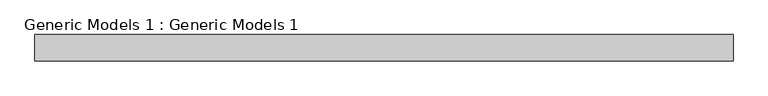
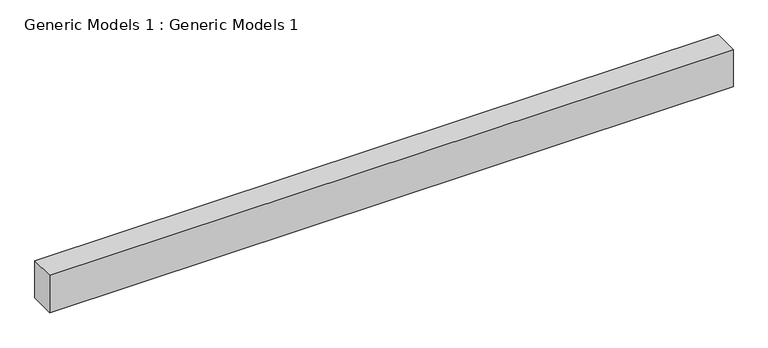
"""IFC4 building model written with IfcOpenShell, lengths in millimetres: proxy geometry, Generic Models 1 : Generic Models 1."""

from ifc_helpers import new_model, si_unit, frame, origin, place, context, project, spatial, polyline, outline, extrude, source, transform, mapped, element, save


def generic_models_1_generic_models_1_ce325797(model_context):
    return source(origin(), model_context, "Body", "SweptSolid", [
        extrude(outline(polyline([(-5171.6277023, -774.0320925), (-11267.6277023, -774.0320925), (-11267.6277023, -545.4320925), (-5171.6277023, -545.4320925), (-5171.6277023, -774.0320925)])), frame((0.0, 0.0, 6400.8), z_axis=(0.0, 0.0, 1.0), x_axis=(1.0, 0.0, 0.0)), (0.0, 0.0, 1.0), 351.4975279),
    ])


if __name__ == "__main__":
    model = new_model("IFC4")
    model_context = context("Model", 3, world=origin())
    ifc_project = project(units=[si_unit("LENGTHUNIT", "METRE", prefix="MILLI")], contexts=[model_context])
    site = spatial("IfcSite", under=ifc_project)
    building = spatial("IfcBuilding", under=site)
    placement = place(None, origin())
    generic_models_1_generic_models_1_shape = generic_models_1_generic_models_1_ce325797(model_context)
    element("IfcBuildingElementProxy", 1, Name="Generic Models 1 : Generic Models 1", ObjectType="Generic Models 1 : Generic Models 1", at=placement, inside=building, context=model_context, shape_type="MappedRepresentation", body=[
        mapped(generic_models_1_generic_models_1_shape, transform((0.0, 0.0, 0.0), x_axis=(1.0, 0.0, 0.0), y_axis=(0.0, 1.0, 0.0), z_axis=(0.0, 0.0, 1.0))),
    ])
    save(model, "model.ifc")

# Revit data of these elements
# Element 1 (IfcBuildingElementProxy, "Generic Models 1 : Generic Models 1")
#   Materials on its faces: "Clad - White"
# Materials
#   "Clad - White": class "Wood", colour RGB 242 242 238, transparency 0, Cost = 0
